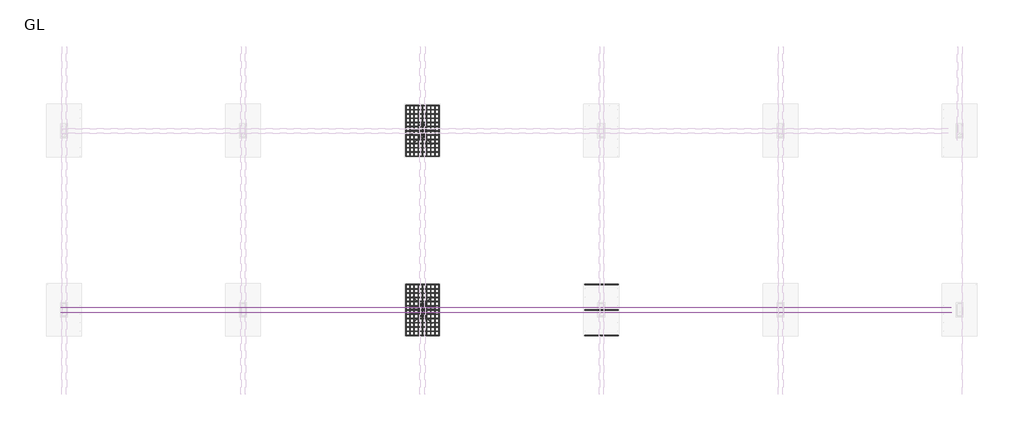
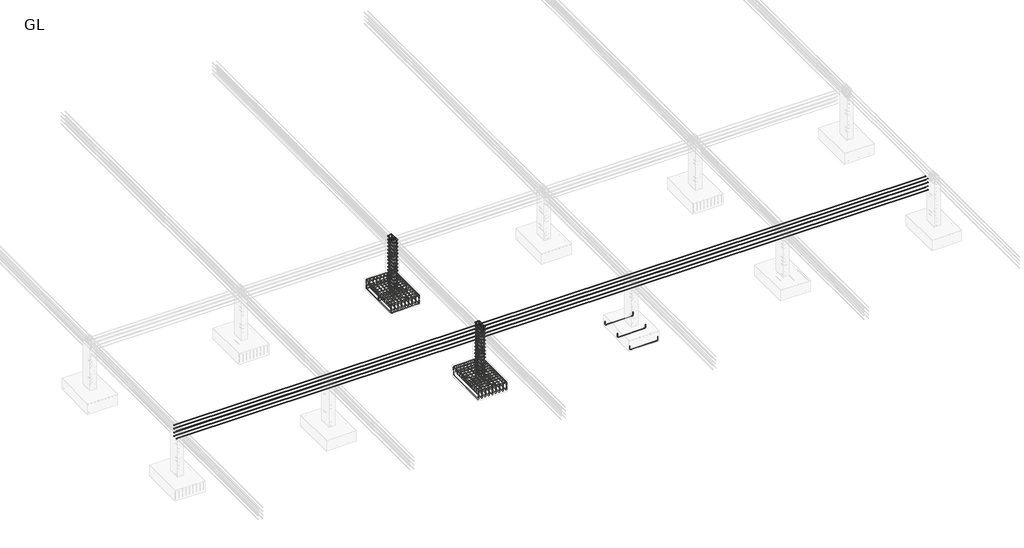
# One storey, part 7 of 16: 22 reinforcing bars.
"""IFC4 building model written with IfcOpenShell, lengths in millimetres."""

from ifc_helpers import new_model, si_unit, point, frame, origin, place, context, project, spatial, polyline, circle_curve, trimmed, segment, composite_curve, source, transform, mapped, element, save
from ifc_brep_helpers import swept_disk

model = new_model("IFC4")

# Units and contexts
model_context = context("Model", 3, world=origin())
ifc_project = project(units=[si_unit("LENGTHUNIT", "METRE", prefix="MILLI")], contexts=[model_context])

# Site, building, storey
site = spatial("IfcSite", under=ifc_project)
building = spatial("IfcBuilding", under=site)
storey = spatial("IfcBuildingStorey", under=building, Name="GL", Elevation=-1829.0)

# Reinforcing bars
placement = place(None, origin())
reinforcing_bar_shape = source(origin(), model_context, "Body", "SolidModel", [
    swept_disk(composite_curve([segment(polyline([(-10050.9544379, -7223.1167521, -2089.0), (-10050.9544379, -7223.1167521, -2213.0)]), True, "CONTINUOUS"), segment(trimmed(circle_curve(frame((-10080.9544379, -7223.1167521, -2213.0), z_axis=(0.0, 1.0, 0.0), x_axis=(30.0, 0.0, 0.0)), 30.0), [point((-10050.9544379, -7223.1167521, -2213.0))], [point((-10080.9544379, -7223.1167521, -2243.0))], True, "CARTESIAN"), True, "CONTINUOUS"), segment(polyline([(-10080.9544379, -7223.1167521, -2243.0), (-11148.9544379, -7223.1167521, -2243.0)]), True, "CONTINUOUS"), segment(trimmed(circle_curve(frame((-11148.9544379, -7223.1167521, -2213.0), z_axis=(0.0, 1.0, 0.0), x_axis=(0.0, 0.0, -30.0)), 30.0), [point((-11148.9544379, -7223.1167521, -2243.0))], [point((-11178.9544379, -7223.1167521, -2213.0))], True, "CARTESIAN"), True, "CONTINUOUS"), segment(polyline([(-11178.9544379, -7223.1167521, -2213.0), (-11178.9544379, -7223.1167521, -2089.0)]), True, "CONTINUOUS")], self_intersect=False), 6.0),
])
element("IfcReinforcingBar", 1, at=placement, inside=storey, context=model_context, shape_type="MappedRepresentation", body=[
    mapped(reinforcing_bar_shape, transform((0.0, 0.0, 0.0), x_axis=(1.0, 0.0, 0.0), y_axis=(0.0, 1.0, 0.0), z_axis=(0.0, 0.0, 1.0))),
    mapped(reinforcing_bar_shape, transform((0.0, -864.0, 0.0), x_axis=(1.0, 0.0, 0.0), y_axis=(0.0, 1.0, 0.0), z_axis=(0.0, 0.0, 1.0))),
    mapped(reinforcing_bar_shape, transform((0.0, -1728.0, 0.0), x_axis=(1.0, 0.0, 0.0), y_axis=(0.0, 1.0, 0.0), z_axis=(0.0, 0.0, 1.0))),
])
reinforcing_bar_2_shape = source(origin(), model_context, "Body", "SolidModel", [
    swept_disk(composite_curve([segment(polyline([(-11178.9544379, -7223.1167521, -2022.436678), (-11178.9544379, -7223.1167521, -1898.436678)]), True, "CONTINUOUS"), segment(trimmed(circle_curve(frame((-11148.9544379, -7223.1167521, -1898.436678), z_axis=(0.0, 1.0, 0.0), x_axis=(-30.0, 0.0, 0.0)), 30.0), [point((-11178.9544379, -7223.1167521, -1898.436678))], [point((-11148.9544379, -7223.1167521, -1868.436678))], True, "CARTESIAN"), True, "CONTINUOUS"), segment(polyline([(-11148.9544379, -7223.1167521, -1868.436678), (-10080.9544379, -7223.1167521, -1868.436678)]), True, "CONTINUOUS"), segment(trimmed(circle_curve(frame((-10080.9544379, -7223.1167521, -1898.436678), z_axis=(0.0, 1.0, 0.0), x_axis=(0.0, 0.0, 30.0)), 30.0), [point((-10080.9544379, -7223.1167521, -1868.436678))], [point((-10050.9544379, -7223.1167521, -1898.436678))], True, "CARTESIAN"), True, "CONTINUOUS"), segment(polyline([(-10050.9544379, -7223.1167521, -1898.436678), (-10050.9544379, -7223.1167521, -2022.436678)]), True, "CONTINUOUS")], self_intersect=False), 6.0),
])
element("IfcReinforcingBar", 2, at=placement, inside=storey, context=model_context, shape_type="MappedRepresentation", body=[
    mapped(reinforcing_bar_2_shape, transform((0.0, 0.0, 0.0), x_axis=(1.0, 0.0, 0.0), y_axis=(0.0, 1.0, 0.0), z_axis=(0.0, 0.0, 1.0))),
    mapped(reinforcing_bar_2_shape, transform((0.0, -144.0, 0.0), x_axis=(1.0, 0.0, 0.0), y_axis=(0.0, 1.0, 0.0), z_axis=(0.0, 0.0, 1.0))),
    mapped(reinforcing_bar_2_shape, transform((0.0, -288.0, 0.0), x_axis=(1.0, 0.0, 0.0), y_axis=(0.0, 1.0, 0.0), z_axis=(0.0, 0.0, 1.0))),
    mapped(reinforcing_bar_2_shape, transform((0.0, -432.0, 0.0), x_axis=(1.0, 0.0, 0.0), y_axis=(0.0, 1.0, 0.0), z_axis=(0.0, 0.0, 1.0))),
    mapped(reinforcing_bar_2_shape, transform((0.0, -576.0, 0.0), x_axis=(1.0, 0.0, 0.0), y_axis=(0.0, 1.0, 0.0), z_axis=(0.0, 0.0, 1.0))),
    mapped(reinforcing_bar_2_shape, transform((0.0, -720.0, 0.0), x_axis=(1.0, 0.0, 0.0), y_axis=(0.0, 1.0, 0.0), z_axis=(0.0, 0.0, 1.0))),
    mapped(reinforcing_bar_2_shape, transform((0.0, -864.0, 0.0), x_axis=(1.0, 0.0, 0.0), y_axis=(0.0, 1.0, 0.0), z_axis=(0.0, 0.0, 1.0))),
    mapped(reinforcing_bar_2_shape, transform((0.0, -1008.0, 0.0), x_axis=(1.0, 0.0, 0.0), y_axis=(0.0, 1.0, 0.0), z_axis=(0.0, 0.0, 1.0))),
    mapped(reinforcing_bar_2_shape, transform((0.0, -1152.0, 0.0), x_axis=(1.0, 0.0, 0.0), y_axis=(0.0, 1.0, 0.0), z_axis=(0.0, 0.0, 1.0))),
    mapped(reinforcing_bar_2_shape, transform((0.0, -1296.0, 0.0), x_axis=(1.0, 0.0, 0.0), y_axis=(0.0, 1.0, 0.0), z_axis=(0.0, 0.0, 1.0))),
    mapped(reinforcing_bar_2_shape, transform((0.0, -1440.0, 0.0), x_axis=(1.0, 0.0, 0.0), y_axis=(0.0, 1.0, 0.0), z_axis=(0.0, 0.0, 1.0))),
    mapped(reinforcing_bar_2_shape, transform((0.0, -1584.0, 0.0), x_axis=(1.0, 0.0, 0.0), y_axis=(0.0, 1.0, 0.0), z_axis=(0.0, 0.0, 1.0))),
    mapped(reinforcing_bar_2_shape, transform((0.0, -1728.0, 0.0), x_axis=(1.0, 0.0, 0.0), y_axis=(0.0, 1.0, 0.0), z_axis=(0.0, 0.0, 1.0))),
])
reinforcing_bar_3_shape = source(origin(), model_context, "Body", "SolidModel", [
    swept_disk(composite_curve([segment(polyline([(-11178.9544379, -8951.1167521, -2027.5081232), (-11178.9544379, -8951.1167521, -1903.5081232)]), True, "CONTINUOUS"), segment(trimmed(circle_curve(frame((-11178.9544379, -8921.1167521, -1903.5081232), z_axis=(-1.0, 0.0, 0.0), x_axis=(0.0, -30.0, 0.0)), 30.0), [point((-11178.9544379, -8951.1167521, -1903.5081232))], [point((-11178.9544379, -8921.1167521, -1873.5081232))], True, "CARTESIAN"), True, "CONTINUOUS"), segment(polyline([(-11178.9544379, -8921.1167521, -1873.5081232), (-11178.9544379, -7253.1167521, -1873.5081232)]), True, "CONTINUOUS"), segment(trimmed(circle_curve(frame((-11178.9544379, -7253.1167521, -1903.5081232), z_axis=(-1.0, 0.0, 0.0), x_axis=(0.0, 0.0, 30.0)), 30.0), [point((-11178.9544379, -7253.1167521, -1873.5081232))], [point((-11178.9544379, -7223.1167521, -1903.5081232))], True, "CARTESIAN"), True, "CONTINUOUS"), segment(polyline([(-11178.9544379, -7223.1167521, -1903.5081232), (-11178.9544379, -7223.1167521, -2027.5081232)]), True, "CONTINUOUS")], self_intersect=False), 6.0),
])
element("IfcReinforcingBar", 3, at=placement, inside=storey, context=model_context, shape_type="MappedRepresentation", body=[
    mapped(reinforcing_bar_3_shape, transform((0.0, 0.0, 0.0), x_axis=(1.0, 0.0, 0.0), y_axis=(0.0, 1.0, 0.0), z_axis=(0.0, 0.0, 1.0))),
    mapped(reinforcing_bar_3_shape, transform((141.0, 0.0, 0.0), x_axis=(1.0, 0.0, 0.0), y_axis=(0.0, 1.0, 0.0), z_axis=(0.0, 0.0, 1.0))),
    mapped(reinforcing_bar_3_shape, transform((282.0, 0.0, 0.0), x_axis=(1.0, 0.0, 0.0), y_axis=(0.0, 1.0, 0.0), z_axis=(0.0, 0.0, 1.0))),
    mapped(reinforcing_bar_3_shape, transform((423.0, 0.0, 0.0), x_axis=(1.0, 0.0, 0.0), y_axis=(0.0, 1.0, 0.0), z_axis=(0.0, 0.0, 1.0))),
    mapped(reinforcing_bar_3_shape, transform((564.0, 0.0, 0.0), x_axis=(1.0, 0.0, 0.0), y_axis=(0.0, 1.0, 0.0), z_axis=(0.0, 0.0, 1.0))),
    mapped(reinforcing_bar_3_shape, transform((705.0, 0.0, 0.0), x_axis=(1.0, 0.0, 0.0), y_axis=(0.0, 1.0, 0.0), z_axis=(0.0, 0.0, 1.0))),
    mapped(reinforcing_bar_3_shape, transform((846.0, 0.0, 0.0), x_axis=(1.0, 0.0, 0.0), y_axis=(0.0, 1.0, 0.0), z_axis=(0.0, 0.0, 1.0))),
    mapped(reinforcing_bar_3_shape, transform((987.0, 0.0, 0.0), x_axis=(1.0, 0.0, 0.0), y_axis=(0.0, 1.0, 0.0), z_axis=(0.0, 0.0, 1.0))),
    mapped(reinforcing_bar_3_shape, transform((1128.0, 0.0, 0.0), x_axis=(1.0, 0.0, 0.0), y_axis=(0.0, 1.0, 0.0), z_axis=(0.0, 0.0, 1.0))),
])
reinforcing_bar_4_shape = source(origin(), model_context, "Body", "SolidModel", [
    swept_disk(composite_curve([segment(polyline([(-10050.9544379, -8951.1167521, -2080.6239909), (-10050.9544379, -8951.1167521, -2204.6239909)]), True, "CONTINUOUS"), segment(trimmed(circle_curve(frame((-10050.9544379, -8921.1167521, -2204.6239909), z_axis=(1.0, 0.0, 0.0), x_axis=(0.0, -30.0, 0.0)), 30.0), [point((-10050.9544379, -8951.1167521, -2204.6239909))], [point((-10050.9544379, -8921.1167521, -2234.6239909))], True, "CARTESIAN"), True, "CONTINUOUS"), segment(polyline([(-10050.9544379, -8921.1167521, -2234.6239909), (-10050.9544379, -7266.1421892, -2234.6239909)]), True, "CONTINUOUS"), segment(trimmed(circle_curve(frame((-10050.9544379, -7266.1421892, -2204.6239909), z_axis=(1.0, 0.0, 0.0), x_axis=(0.0, 0.0, -30.0)), 30.0), [point((-10050.9544379, -7266.1421892, -2234.6239909))], [point((-10050.9544379, -7236.1421892, -2204.6239909))], True, "CARTESIAN"), True, "CONTINUOUS"), segment(polyline([(-10050.9544379, -7236.1421892, -2204.6239909), (-10050.9544379, -7236.1421892, -2080.6239909)]), True, "CONTINUOUS")], self_intersect=False), 6.0),
])
element("IfcReinforcingBar", 4, at=placement, inside=storey, context=model_context, shape_type="MappedRepresentation", body=[
    mapped(reinforcing_bar_4_shape, transform((0.0, 0.0, 0.0), x_axis=(1.0, 0.0, 0.0), y_axis=(0.0, 1.0, 0.0), z_axis=(0.0, 0.0, 1.0))),
    mapped(reinforcing_bar_4_shape, transform((-141.0, 0.0, 0.0), x_axis=(1.0, 0.0, 0.0), y_axis=(0.0, 1.0, 0.0), z_axis=(0.0, 0.0, 1.0))),
    mapped(reinforcing_bar_4_shape, transform((-282.0, 0.0, 0.0), x_axis=(1.0, 0.0, 0.0), y_axis=(0.0, 1.0, 0.0), z_axis=(0.0, 0.0, 1.0))),
    mapped(reinforcing_bar_4_shape, transform((-423.0, 0.0, 0.0), x_axis=(1.0, 0.0, 0.0), y_axis=(0.0, 1.0, 0.0), z_axis=(0.0, 0.0, 1.0))),
    mapped(reinforcing_bar_4_shape, transform((-564.0, 0.0, 0.0), x_axis=(1.0, 0.0, 0.0), y_axis=(0.0, 1.0, 0.0), z_axis=(0.0, 0.0, 1.0))),
    mapped(reinforcing_bar_4_shape, transform((-705.0, 0.0, 0.0), x_axis=(1.0, 0.0, 0.0), y_axis=(0.0, 1.0, 0.0), z_axis=(0.0, 0.0, 1.0))),
    mapped(reinforcing_bar_4_shape, transform((-846.0, 0.0, 0.0), x_axis=(1.0, 0.0, 0.0), y_axis=(0.0, 1.0, 0.0), z_axis=(0.0, 0.0, 1.0))),
    mapped(reinforcing_bar_4_shape, transform((-987.0, 0.0, 0.0), x_axis=(1.0, 0.0, 0.0), y_axis=(0.0, 1.0, 0.0), z_axis=(0.0, 0.0, 1.0))),
    mapped(reinforcing_bar_4_shape, transform((-1128.0, 0.0, 0.0), x_axis=(1.0, 0.0, 0.0), y_axis=(0.0, 1.0, 0.0), z_axis=(0.0, 0.0, 1.0))),
])
reinforcing_bar_5_shape = source(origin(), model_context, "Body", "SolidModel", [
    swept_disk(composite_curve([segment(polyline([(-3954.9544379, -13319.1167521, -2089.0), (-3954.9544379, -13319.1167521, -2213.0)]), True, "CONTINUOUS"), segment(trimmed(circle_curve(frame((-3984.9544379, -13319.1167521, -2213.0), z_axis=(0.0, 1.0, 0.0), x_axis=(30.0, 0.0, 0.0)), 30.0), [point((-3954.9544379, -13319.1167521, -2213.0))], [point((-3984.9544379, -13319.1167521, -2243.0))], True, "CARTESIAN"), True, "CONTINUOUS"), segment(polyline([(-3984.9544379, -13319.1167521, -2243.0), (-5052.9544379, -13319.1167521, -2243.0)]), True, "CONTINUOUS"), segment(trimmed(circle_curve(frame((-5052.9544379, -13319.1167521, -2213.0), z_axis=(0.0, 1.0, 0.0), x_axis=(0.0, 0.0, -30.0)), 30.0), [point((-5052.9544379, -13319.1167521, -2243.0))], [point((-5082.9544379, -13319.1167521, -2213.0))], True, "CARTESIAN"), True, "CONTINUOUS"), segment(polyline([(-5082.9544379, -13319.1167521, -2213.0), (-5082.9544379, -13319.1167521, -2089.0)]), True, "CONTINUOUS")], self_intersect=False), 6.0),
])
element("IfcReinforcingBar", 5, at=placement, inside=storey, context=model_context, shape_type="MappedRepresentation", body=[
    mapped(reinforcing_bar_5_shape, transform((0.0, 0.0, 0.0), x_axis=(1.0, 0.0, 0.0), y_axis=(0.0, 1.0, 0.0), z_axis=(0.0, 0.0, 1.0))),
    mapped(reinforcing_bar_5_shape, transform((0.0, -864.0, 0.0), x_axis=(1.0, 0.0, 0.0), y_axis=(0.0, 1.0, 0.0), z_axis=(0.0, 0.0, 1.0))),
    mapped(reinforcing_bar_5_shape, transform((0.0, -1728.0, 0.0), x_axis=(1.0, 0.0, 0.0), y_axis=(0.0, 1.0, 0.0), z_axis=(0.0, 0.0, 1.0))),
])
reinforcing_bar_6_shape = source(origin(), model_context, "Body", "SolidModel", [
    swept_disk(composite_curve([segment(polyline([(-11178.9544379, -13319.1167521, -2022.436678), (-11178.9544379, -13319.1167521, -1898.436678)]), True, "CONTINUOUS"), segment(trimmed(circle_curve(frame((-11148.9544379, -13319.1167521, -1898.436678), z_axis=(0.0, 1.0, 0.0), x_axis=(-30.0, 0.0, 0.0)), 30.0), [point((-11178.9544379, -13319.1167521, -1898.436678))], [point((-11148.9544379, -13319.1167521, -1868.436678))], True, "CARTESIAN"), True, "CONTINUOUS"), segment(polyline([(-11148.9544379, -13319.1167521, -1868.436678), (-10080.9544379, -13319.1167521, -1868.436678)]), True, "CONTINUOUS"), segment(trimmed(circle_curve(frame((-10080.9544379, -13319.1167521, -1898.436678), z_axis=(0.0, 1.0, 0.0), x_axis=(0.0, 0.0, 30.0)), 30.0), [point((-10080.9544379, -13319.1167521, -1868.436678))], [point((-10050.9544379, -13319.1167521, -1898.436678))], True, "CARTESIAN"), True, "CONTINUOUS"), segment(polyline([(-10050.9544379, -13319.1167521, -1898.436678), (-10050.9544379, -13319.1167521, -2022.436678)]), True, "CONTINUOUS")], self_intersect=False), 6.0),
])
element("IfcReinforcingBar", 6, at=placement, inside=storey, context=model_context, shape_type="MappedRepresentation", body=[
    mapped(reinforcing_bar_6_shape, transform((0.0, 0.0, 0.0), x_axis=(1.0, 0.0, 0.0), y_axis=(0.0, 1.0, 0.0), z_axis=(0.0, 0.0, 1.0))),
    mapped(reinforcing_bar_6_shape, transform((0.0, -144.0, 0.0), x_axis=(1.0, 0.0, 0.0), y_axis=(0.0, 1.0, 0.0), z_axis=(0.0, 0.0, 1.0))),
    mapped(reinforcing_bar_6_shape, transform((0.0, -288.0, 0.0), x_axis=(1.0, 0.0, 0.0), y_axis=(0.0, 1.0, 0.0), z_axis=(0.0, 0.0, 1.0))),
    mapped(reinforcing_bar_6_shape, transform((0.0, -432.0, 0.0), x_axis=(1.0, 0.0, 0.0), y_axis=(0.0, 1.0, 0.0), z_axis=(0.0, 0.0, 1.0))),
    mapped(reinforcing_bar_6_shape, transform((0.0, -576.0, 0.0), x_axis=(1.0, 0.0, 0.0), y_axis=(0.0, 1.0, 0.0), z_axis=(0.0, 0.0, 1.0))),
    mapped(reinforcing_bar_6_shape, transform((0.0, -720.0, 0.0), x_axis=(1.0, 0.0, 0.0), y_axis=(0.0, 1.0, 0.0), z_axis=(0.0, 0.0, 1.0))),
    mapped(reinforcing_bar_6_shape, transform((0.0, -864.0, 0.0), x_axis=(1.0, 0.0, 0.0), y_axis=(0.0, 1.0, 0.0), z_axis=(0.0, 0.0, 1.0))),
    mapped(reinforcing_bar_6_shape, transform((0.0, -1008.0, 0.0), x_axis=(1.0, 0.0, 0.0), y_axis=(0.0, 1.0, 0.0), z_axis=(0.0, 0.0, 1.0))),
    mapped(reinforcing_bar_6_shape, transform((0.0, -1152.0, 0.0), x_axis=(1.0, 0.0, 0.0), y_axis=(0.0, 1.0, 0.0), z_axis=(0.0, 0.0, 1.0))),
    mapped(reinforcing_bar_6_shape, transform((0.0, -1296.0, 0.0), x_axis=(1.0, 0.0, 0.0), y_axis=(0.0, 1.0, 0.0), z_axis=(0.0, 0.0, 1.0))),
    mapped(reinforcing_bar_6_shape, transform((0.0, -1440.0, 0.0), x_axis=(1.0, 0.0, 0.0), y_axis=(0.0, 1.0, 0.0), z_axis=(0.0, 0.0, 1.0))),
    mapped(reinforcing_bar_6_shape, transform((0.0, -1584.0, 0.0), x_axis=(1.0, 0.0, 0.0), y_axis=(0.0, 1.0, 0.0), z_axis=(0.0, 0.0, 1.0))),
    mapped(reinforcing_bar_6_shape, transform((0.0, -1728.0, 0.0), x_axis=(1.0, 0.0, 0.0), y_axis=(0.0, 1.0, 0.0), z_axis=(0.0, 0.0, 1.0))),
])
reinforcing_bar_7_shape = source(origin(), model_context, "Body", "SolidModel", [
    swept_disk(composite_curve([segment(polyline([(-11178.9544379, -15047.1167521, -2027.5081232), (-11178.9544379, -15047.1167521, -1903.5081232)]), True, "CONTINUOUS"), segment(trimmed(circle_curve(frame((-11178.9544379, -15017.1167521, -1903.5081232), z_axis=(-1.0, 0.0, 0.0), x_axis=(0.0, -30.0, 0.0)), 30.0), [point((-11178.9544379, -15047.1167521, -1903.5081232))], [point((-11178.9544379, -15017.1167521, -1873.5081232))], True, "CARTESIAN"), True, "CONTINUOUS"), segment(polyline([(-11178.9544379, -15017.1167521, -1873.5081232), (-11178.9544379, -13349.1167521, -1873.5081232)]), True, "CONTINUOUS"), segment(trimmed(circle_curve(frame((-11178.9544379, -13349.1167521, -1903.5081232), z_axis=(-1.0, 0.0, 0.0), x_axis=(0.0, 0.0, 30.0)), 30.0), [point((-11178.9544379, -13349.1167521, -1873.5081232))], [point((-11178.9544379, -13319.1167521, -1903.5081232))], True, "CARTESIAN"), True, "CONTINUOUS"), segment(polyline([(-11178.9544379, -13319.1167521, -1903.5081232), (-11178.9544379, -13319.1167521, -2027.5081232)]), True, "CONTINUOUS")], self_intersect=False), 6.0),
])
element("IfcReinforcingBar", 7, at=placement, inside=storey, context=model_context, shape_type="MappedRepresentation", body=[
    mapped(reinforcing_bar_7_shape, transform((0.0, 0.0, 0.0), x_axis=(1.0, 0.0, 0.0), y_axis=(0.0, 1.0, 0.0), z_axis=(0.0, 0.0, 1.0))),
    mapped(reinforcing_bar_7_shape, transform((141.0, 0.0, 0.0), x_axis=(1.0, 0.0, 0.0), y_axis=(0.0, 1.0, 0.0), z_axis=(0.0, 0.0, 1.0))),
    mapped(reinforcing_bar_7_shape, transform((282.0, 0.0, 0.0), x_axis=(1.0, 0.0, 0.0), y_axis=(0.0, 1.0, 0.0), z_axis=(0.0, 0.0, 1.0))),
    mapped(reinforcing_bar_7_shape, transform((423.0, 0.0, 0.0), x_axis=(1.0, 0.0, 0.0), y_axis=(0.0, 1.0, 0.0), z_axis=(0.0, 0.0, 1.0))),
    mapped(reinforcing_bar_7_shape, transform((564.0, 0.0, 0.0), x_axis=(1.0, 0.0, 0.0), y_axis=(0.0, 1.0, 0.0), z_axis=(0.0, 0.0, 1.0))),
    mapped(reinforcing_bar_7_shape, transform((705.0, 0.0, 0.0), x_axis=(1.0, 0.0, 0.0), y_axis=(0.0, 1.0, 0.0), z_axis=(0.0, 0.0, 1.0))),
    mapped(reinforcing_bar_7_shape, transform((846.0, 0.0, 0.0), x_axis=(1.0, 0.0, 0.0), y_axis=(0.0, 1.0, 0.0), z_axis=(0.0, 0.0, 1.0))),
    mapped(reinforcing_bar_7_shape, transform((987.0, 0.0, 0.0), x_axis=(1.0, 0.0, 0.0), y_axis=(0.0, 1.0, 0.0), z_axis=(0.0, 0.0, 1.0))),
    mapped(reinforcing_bar_7_shape, transform((1128.0, 0.0, 0.0), x_axis=(1.0, 0.0, 0.0), y_axis=(0.0, 1.0, 0.0), z_axis=(0.0, 0.0, 1.0))),
])
reinforcing_bar_8_shape = source(origin(), model_context, "Body", "SolidModel", [
    swept_disk(composite_curve([segment(polyline([(-10050.9544379, -15047.1167521, -2080.6239909), (-10050.9544379, -15047.1167521, -2204.6239909)]), True, "CONTINUOUS"), segment(trimmed(circle_curve(frame((-10050.9544379, -15017.1167521, -2204.6239909), z_axis=(1.0, 0.0, 0.0), x_axis=(0.0, -30.0, 0.0)), 30.0), [point((-10050.9544379, -15047.1167521, -2204.6239909))], [point((-10050.9544379, -15017.1167521, -2234.6239909))], True, "CARTESIAN"), True, "CONTINUOUS"), segment(polyline([(-10050.9544379, -15017.1167521, -2234.6239909), (-10050.9544379, -13362.1421892, -2234.6239909)]), True, "CONTINUOUS"), segment(trimmed(circle_curve(frame((-10050.9544379, -13362.1421892, -2204.6239909), z_axis=(1.0, 0.0, 0.0), x_axis=(0.0, 0.0, -30.0)), 30.0), [point((-10050.9544379, -13362.1421892, -2234.6239909))], [point((-10050.9544379, -13332.1421892, -2204.6239909))], True, "CARTESIAN"), True, "CONTINUOUS"), segment(polyline([(-10050.9544379, -13332.1421892, -2204.6239909), (-10050.9544379, -13332.1421892, -2080.6239909)]), True, "CONTINUOUS")], self_intersect=False), 6.0),
])
element("IfcReinforcingBar", 8, at=placement, inside=storey, context=model_context, shape_type="MappedRepresentation", body=[
    mapped(reinforcing_bar_8_shape, transform((0.0, 0.0, 0.0), x_axis=(1.0, 0.0, 0.0), y_axis=(0.0, 1.0, 0.0), z_axis=(0.0, 0.0, 1.0))),
    mapped(reinforcing_bar_8_shape, transform((-141.0, 0.0, 0.0), x_axis=(1.0, 0.0, 0.0), y_axis=(0.0, 1.0, 0.0), z_axis=(0.0, 0.0, 1.0))),
    mapped(reinforcing_bar_8_shape, transform((-282.0, 0.0, 0.0), x_axis=(1.0, 0.0, 0.0), y_axis=(0.0, 1.0, 0.0), z_axis=(0.0, 0.0, 1.0))),
    mapped(reinforcing_bar_8_shape, transform((-423.0, 0.0, 0.0), x_axis=(1.0, 0.0, 0.0), y_axis=(0.0, 1.0, 0.0), z_axis=(0.0, 0.0, 1.0))),
    mapped(reinforcing_bar_8_shape, transform((-564.0, 0.0, 0.0), x_axis=(1.0, 0.0, 0.0), y_axis=(0.0, 1.0, 0.0), z_axis=(0.0, 0.0, 1.0))),
    mapped(reinforcing_bar_8_shape, transform((-705.0, 0.0, 0.0), x_axis=(1.0, 0.0, 0.0), y_axis=(0.0, 1.0, 0.0), z_axis=(0.0, 0.0, 1.0))),
    mapped(reinforcing_bar_8_shape, transform((-846.0, 0.0, 0.0), x_axis=(1.0, 0.0, 0.0), y_axis=(0.0, 1.0, 0.0), z_axis=(0.0, 0.0, 1.0))),
    mapped(reinforcing_bar_8_shape, transform((-987.0, 0.0, 0.0), x_axis=(1.0, 0.0, 0.0), y_axis=(0.0, 1.0, 0.0), z_axis=(0.0, 0.0, 1.0))),
    mapped(reinforcing_bar_8_shape, transform((-1128.0, 0.0, 0.0), x_axis=(1.0, 0.0, 0.0), y_axis=(0.0, 1.0, 0.0), z_axis=(0.0, 0.0, 1.0))),
])
reinforcing_bar_9_shape = source(origin(), model_context, "Body", "SolidModel", [
    swept_disk(composite_curve([segment(polyline([(-10607.4864005, -14258.2223078, -1793.0), (-10695.1676414, -14345.9035486, -1793.0)]), True, "CONTINUOUS"), segment(trimmed(circle_curve(frame((-10673.9544379, -14367.1167521, -1793.0), z_axis=(0.0, 0.0, 1.0), x_axis=(-21.21320349999951, 21.213203500001327, 0.0)), 30.0), [point((-10695.1676414, -14345.9035486, -1793.0))], [point((-10673.9544379, -14397.1167521, -1793.0))], True, "CARTESIAN"), True, "CONTINUOUS"), segment(polyline([(-10673.9544379, -14397.1167521, -1793.0), (-10555.9544379, -14397.1167521, -1793.0)]), True, "CONTINUOUS"), segment(trimmed(circle_curve(frame((-10555.9544379, -14367.1167521, -1793.0), z_axis=(0.0, 0.0, 1.0), x_axis=(0.0, -30.0, 0.0)), 30.0), [point((-10555.9544379, -14397.1167521, -1793.0))], [point((-10525.9544379, -14367.1167521, -1793.0))], True, "CARTESIAN"), True, "CONTINUOUS"), segment(polyline([(-10525.9544379, -14367.1167521, -1793.0), (-10525.9544379, -13999.1167521, -1793.0)]), True, "CONTINUOUS"), segment(trimmed(circle_curve(frame((-10555.8864962, -13999.1167521, -1795.0178916), z_axis=(-0.06726305234213417, 0.0, 0.9977352764083365), x_axis=(29.93205830000079, 0.0, 2.0178915999999845)), 30.0), [point((-10525.9544379, -13999.1167521, -1793.0))], [point((-10555.8864962, -13969.1167521, -1795.0178916))], True, "CARTESIAN"), True, "CONTINUOUS"), segment(polyline([(-10555.8864962, -13969.1167521, -1795.0178916), (-10674.0223796, -13969.1167521, -1802.9821084)]), True, "CONTINUOUS"), segment(trimmed(circle_curve(frame((-10674.0223796, -13999.1167521, -1802.9821084), z_axis=(-0.06726305234213417, 0.0, 0.9977352764083365), x_axis=(0.0, 30.0, 0.0)), 30.0), [point((-10674.0223796, -13969.1167521, -1802.9821084))], [point((-10703.9544379, -13999.1167521, -1805.0))], True, "CARTESIAN"), True, "CONTINUOUS"), segment(polyline([(-10703.9544379, -13999.1167521, -1805.0), (-10703.9544379, -14367.1167521, -1805.0)]), True, "CONTINUOUS"), segment(trimmed(circle_curve(frame((-10673.9544379, -14367.1167521, -1805.0), z_axis=(0.0, 0.0, 1.0), x_axis=(-30.0, 0.0, 0.0)), 30.0), [point((-10703.9544379, -14367.1167521, -1805.0))], [point((-10652.7412345, -14388.3299555, -1805.0))], True, "CARTESIAN"), True, "CONTINUOUS"), segment(polyline([(-10652.7412345, -14388.3299555, -1805.0), (-10565.0599936, -14300.6487146, -1805.0)]), True, "CONTINUOUS")], self_intersect=False), 6.0),
])
element("IfcReinforcingBar", 9, at=placement, inside=storey, context=model_context, shape_type="MappedRepresentation", body=[
    mapped(reinforcing_bar_9_shape, transform((0.0, 0.0, 0.0), x_axis=(1.0, 0.0, 0.0), y_axis=(0.0, 1.0, 0.0), z_axis=(0.0, 0.0, 1.0))),
    mapped(reinforcing_bar_9_shape, transform((0.0, 0.0, 144.8571429), x_axis=(1.0, 0.0, 0.0), y_axis=(0.0, 1.0, 0.0), z_axis=(0.0, 0.0, 1.0))),
    mapped(reinforcing_bar_9_shape, transform((0.0, 0.0, 289.7142857), x_axis=(1.0, 0.0, 0.0), y_axis=(0.0, 1.0, 0.0), z_axis=(0.0, 0.0, 1.0))),
    mapped(reinforcing_bar_9_shape, transform((0.0, 0.0, 434.5714286), x_axis=(1.0, 0.0, 0.0), y_axis=(0.0, 1.0, 0.0), z_axis=(0.0, 0.0, 1.0))),
    mapped(reinforcing_bar_9_shape, transform((0.0, 0.0, 579.4285714), x_axis=(1.0, 0.0, 0.0), y_axis=(0.0, 1.0, 0.0), z_axis=(0.0, 0.0, 1.0))),
    mapped(reinforcing_bar_9_shape, transform((0.0, 0.0, 724.2857143), x_axis=(1.0, 0.0, 0.0), y_axis=(0.0, 1.0, 0.0), z_axis=(0.0, 0.0, 1.0))),
    mapped(reinforcing_bar_9_shape, transform((0.0, 0.0, 869.1428571), x_axis=(1.0, 0.0, 0.0), y_axis=(0.0, 1.0, 0.0), z_axis=(0.0, 0.0, 1.0))),
    mapped(reinforcing_bar_9_shape, transform((0.0, 0.0, 1014.0), x_axis=(1.0, 0.0, 0.0), y_axis=(0.0, 1.0, 0.0), z_axis=(0.0, 0.0, 1.0))),
    mapped(reinforcing_bar_9_shape, transform((0.0, 0.0, 1158.8571429), x_axis=(1.0, 0.0, 0.0), y_axis=(0.0, 1.0, 0.0), z_axis=(0.0, 0.0, 1.0))),
    mapped(reinforcing_bar_9_shape, transform((0.0, 0.0, 1303.7142857), x_axis=(1.0, 0.0, 0.0), y_axis=(0.0, 1.0, 0.0), z_axis=(0.0, 0.0, 1.0))),
    mapped(reinforcing_bar_9_shape, transform((0.0, 0.0, 1448.5714286), x_axis=(1.0, 0.0, 0.0), y_axis=(0.0, 1.0, 0.0), z_axis=(0.0, 0.0, 1.0))),
    mapped(reinforcing_bar_9_shape, transform((0.0, 0.0, 1593.4285714), x_axis=(1.0, 0.0, 0.0), y_axis=(0.0, 1.0, 0.0), z_axis=(0.0, 0.0, 1.0))),
    mapped(reinforcing_bar_9_shape, transform((0.0, 0.0, 1738.2857143), x_axis=(1.0, 0.0, 0.0), y_axis=(0.0, 1.0, 0.0), z_axis=(0.0, 0.0, 1.0))),
    mapped(reinforcing_bar_9_shape, transform((0.0, 0.0, 1883.1428571), x_axis=(1.0, 0.0, 0.0), y_axis=(0.0, 1.0, 0.0), z_axis=(0.0, 0.0, 1.0))),
    mapped(reinforcing_bar_9_shape, transform((0.0, 0.0, 2028.0), x_axis=(1.0, 0.0, 0.0), y_axis=(0.0, 1.0, 0.0), z_axis=(0.0, 0.0, 1.0))),
])
element("IfcReinforcingBar", 10, at=placement, inside=storey, context=model_context, shape_type="SolidModel", body=[
    swept_disk(composite_curve([segment(polyline([(-10672.0642232, -14368.0642439, 241.0), (-10672.0642232, -14368.0642439, -2129.0)]), True, "CONTINUOUS"), segment(trimmed(circle_curve(frame((-10693.2774266, -14389.2774473, -2129.0), z_axis=(-0.7071067811865187, 0.7071067811865764, 0.0), x_axis=(21.213203400000566, 21.213203400000566, 0.0)), 30.0), [point((-10672.0642232, -14368.0642439, -2129.0))], [point((-10693.2774266, -14389.2774473, -2159.0))], True, "CARTESIAN"), True, "CONTINUOUS"), segment(polyline([(-10693.2774266, -14389.2774473, -2159.0), (-10940.7648, -14636.7648207, -2159.0)]), True, "CONTINUOUS")], self_intersect=False), 6.0),
])
element("IfcReinforcingBar", 11, at=placement, inside=storey, context=model_context, shape_type="SolidModel", body=[
    swept_disk(composite_curve([segment(polyline([(-10672.0642232, -13998.1692603, 241.0), (-10672.0642232, -13998.1692603, -2129.0)]), True, "CONTINUOUS"), segment(trimmed(circle_curve(frame((-10693.2774266, -13976.9560568, -2129.0), z_axis=(0.7071067811865218, 0.7071067811865733, 0.0), x_axis=(21.213203400000566, -21.21320349999951, 0.0)), 30.0), [point((-10672.0642232, -13998.1692603, -2129.0))], [point((-10693.2774266, -13976.9560568, -2159.0))], True, "CARTESIAN"), True, "CONTINUOUS"), segment(polyline([(-10693.2774266, -13976.9560568, -2159.0), (-10940.7648, -13729.4686834, -2159.0)]), True, "CONTINUOUS")], self_intersect=False), 6.0),
])
element("IfcReinforcingBar", 12, at=placement, inside=storey, context=model_context, shape_type="SolidModel", body=[
    swept_disk(composite_curve([segment(polyline([(-10557.8446527, -14368.0642439, 241.0), (-10557.8446527, -14368.0642439, -2129.0)]), True, "CONTINUOUS"), segment(trimmed(circle_curve(frame((-10536.6314492, -14389.2774473, -2129.0), z_axis=(-0.7071067811865248, -0.7071067811865703, 0.0), x_axis=(-21.21320349999951, 21.213203400000566, 0.0)), 30.0), [point((-10557.8446527, -14368.0642439, -2129.0))], [point((-10536.6314492, -14389.2774473, -2159.0))], True, "CARTESIAN"), True, "CONTINUOUS"), segment(polyline([(-10536.6314492, -14389.2774473, -2159.0), (-10289.1440758, -14636.7648207, -2159.0)]), True, "CONTINUOUS")], self_intersect=False), 6.0),
])
element("IfcReinforcingBar", 13, at=placement, inside=storey, context=model_context, shape_type="SolidModel", body=[
    swept_disk(composite_curve([segment(polyline([(-10557.8446527, -13998.1692603, 241.0), (-10557.8446527, -13998.1692603, -2129.0)]), True, "CONTINUOUS"), segment(trimmed(circle_curve(frame((-10536.6314492, -13976.9560568, -2129.0), z_axis=(0.7071067811865157, -0.7071067811865794, 0.0), x_axis=(-21.21320349999951, -21.21320349999951, 0.0)), 30.0), [point((-10557.8446527, -13998.1692603, -2129.0))], [point((-10536.6314492, -13976.9560568, -2159.0))], True, "CARTESIAN"), True, "CONTINUOUS"), segment(polyline([(-10536.6314492, -13976.9560568, -2159.0), (-10289.1440758, -13729.4686834, -2159.0)]), True, "CONTINUOUS")], self_intersect=False), 6.0),
])
reinforcing_bar_10_shape = source(origin(), model_context, "Body", "SolidModel", [
    swept_disk(composite_curve([segment(polyline([(-10672.0642232, -14290.9117405, 241.0), (-10672.0642232, -14290.9117405, -2129.0)]), True, "CONTINUOUS"), segment(trimmed(circle_curve(frame((-10702.0642232, -14290.9117405, -2129.0), z_axis=(0.0, 1.0, 0.0), x_axis=(30.0, 0.0, 0.0)), 30.0), [point((-10672.0642232, -14290.9117405, -2129.0))], [point((-10702.0642232, -14290.9117405, -2159.0))], True, "CARTESIAN"), True, "CONTINUOUS"), segment(polyline([(-10702.0642232, -14290.9117405, -2159.0), (-11052.0642232, -14290.9117405, -2159.0)]), True, "CONTINUOUS")], self_intersect=False), 6.0),
])
element("IfcReinforcingBar", 14, at=placement, inside=storey, context=model_context, shape_type="MappedRepresentation", body=[
    mapped(reinforcing_bar_10_shape, transform((0.0, 0.0, 0.0), x_axis=(1.0, 0.0, 0.0), y_axis=(0.0, 1.0, 0.0), z_axis=(0.0, 0.0, 1.0))),
    mapped(reinforcing_bar_10_shape, transform((0.0, 123.5823926, 0.0), x_axis=(1.0, 0.0, 0.0), y_axis=(0.0, 1.0, 0.0), z_axis=(0.0, 0.0, 1.0))),
    mapped(reinforcing_bar_10_shape, transform((0.0, 247.1647853, 0.0), x_axis=(1.0, 0.0, 0.0), y_axis=(0.0, 1.0, 0.0), z_axis=(0.0, 0.0, 1.0))),
])
reinforcing_bar_11_shape = source(origin(), model_context, "Body", "SolidModel", [
    swept_disk(composite_curve([segment(polyline([(-10557.8446527, -14290.9117405, 241.0), (-10557.8446527, -14290.9117405, -2129.0)]), True, "CONTINUOUS"), segment(trimmed(circle_curve(frame((-10527.8446527, -14290.9117405, -2129.0), z_axis=(0.0, -1.0, 0.0), x_axis=(-30.0, 0.0, 0.0)), 30.0), [point((-10557.8446527, -14290.9117405, -2129.0))], [point((-10527.8446527, -14290.9117405, -2159.0))], True, "CARTESIAN"), True, "CONTINUOUS"), segment(polyline([(-10527.8446527, -14290.9117405, -2159.0), (-10177.8446527, -14290.9117405, -2159.0)]), True, "CONTINUOUS")], self_intersect=False), 6.0),
])
element("IfcReinforcingBar", 15, at=placement, inside=storey, context=model_context, shape_type="MappedRepresentation", body=[
    mapped(reinforcing_bar_11_shape, transform((0.0, 0.0, 0.0), x_axis=(1.0, 0.0, 0.0), y_axis=(0.0, 1.0, 0.0), z_axis=(0.0, 0.0, 1.0))),
    mapped(reinforcing_bar_11_shape, transform((0.0, 123.5823926, 0.0), x_axis=(1.0, 0.0, 0.0), y_axis=(0.0, 1.0, 0.0), z_axis=(0.0, 0.0, 1.0))),
    mapped(reinforcing_bar_11_shape, transform((0.0, 247.1647853, 0.0), x_axis=(1.0, 0.0, 0.0), y_axis=(0.0, 1.0, 0.0), z_axis=(0.0, 0.0, 1.0))),
])
reinforcing_bar_12_shape = source(origin(), model_context, "Body", "SolidModel", [
    swept_disk(composite_curve([segment(polyline([(-10607.4864005, -8162.2223078, -1793.0), (-10695.1676414, -8249.9035486, -1793.0)]), True, "CONTINUOUS"), segment(trimmed(circle_curve(frame((-10673.9544379, -8271.1167521, -1793.0), z_axis=(0.0, 0.0, 1.0), x_axis=(-21.21320349999951, 21.213203500001327, 0.0)), 30.0), [point((-10695.1676414, -8249.9035486, -1793.0))], [point((-10673.9544379, -8301.1167521, -1793.0))], True, "CARTESIAN"), True, "CONTINUOUS"), segment(polyline([(-10673.9544379, -8301.1167521, -1793.0), (-10555.9544379, -8301.1167521, -1793.0)]), True, "CONTINUOUS"), segment(trimmed(circle_curve(frame((-10555.9544379, -8271.1167521, -1793.0), z_axis=(0.0, 0.0, 1.0), x_axis=(0.0, -30.0, 0.0)), 30.0), [point((-10555.9544379, -8301.1167521, -1793.0))], [point((-10525.9544379, -8271.1167521, -1793.0))], True, "CARTESIAN"), True, "CONTINUOUS"), segment(polyline([(-10525.9544379, -8271.1167521, -1793.0), (-10525.9544379, -7903.1167521, -1793.0)]), True, "CONTINUOUS"), segment(trimmed(circle_curve(frame((-10555.8864962, -7903.1167521, -1795.0178916), z_axis=(-0.06726305234213417, 0.0, 0.9977352764083365), x_axis=(29.93205830000079, 0.0, 2.0178915999999845)), 30.0), [point((-10525.9544379, -7903.1167521, -1793.0))], [point((-10555.8864962, -7873.1167521, -1795.0178916))], True, "CARTESIAN"), True, "CONTINUOUS"), segment(polyline([(-10555.8864962, -7873.1167521, -1795.0178916), (-10674.0223796, -7873.1167521, -1802.9821084)]), True, "CONTINUOUS"), segment(trimmed(circle_curve(frame((-10674.0223796, -7903.1167521, -1802.9821084), z_axis=(-0.06726305234213417, 0.0, 0.9977352764083365), x_axis=(0.0, 30.0, 0.0)), 30.0), [point((-10674.0223796, -7873.1167521, -1802.9821084))], [point((-10703.9544379, -7903.1167521, -1805.0))], True, "CARTESIAN"), True, "CONTINUOUS"), segment(polyline([(-10703.9544379, -7903.1167521, -1805.0), (-10703.9544379, -8271.1167521, -1805.0)]), True, "CONTINUOUS"), segment(trimmed(circle_curve(frame((-10673.9544379, -8271.1167521, -1805.0), z_axis=(0.0, 0.0, 1.0), x_axis=(-30.0, 0.0, 0.0)), 30.0), [point((-10703.9544379, -8271.1167521, -1805.0))], [point((-10652.7412345, -8292.3299555, -1805.0))], True, "CARTESIAN"), True, "CONTINUOUS"), segment(polyline([(-10652.7412345, -8292.3299555, -1805.0), (-10565.0599936, -8204.6487146, -1805.0)]), True, "CONTINUOUS")], self_intersect=False), 6.0),
])
element("IfcReinforcingBar", 16, at=placement, inside=storey, context=model_context, shape_type="MappedRepresentation", body=[
    mapped(reinforcing_bar_12_shape, transform((0.0, 0.0, 0.0), x_axis=(1.0, 0.0, 0.0), y_axis=(0.0, 1.0, 0.0), z_axis=(0.0, 0.0, 1.0))),
    mapped(reinforcing_bar_12_shape, transform((0.0, 0.0, 144.8571429), x_axis=(1.0, 0.0, 0.0), y_axis=(0.0, 1.0, 0.0), z_axis=(0.0, 0.0, 1.0))),
    mapped(reinforcing_bar_12_shape, transform((0.0, 0.0, 289.7142857), x_axis=(1.0, 0.0, 0.0), y_axis=(0.0, 1.0, 0.0), z_axis=(0.0, 0.0, 1.0))),
    mapped(reinforcing_bar_12_shape, transform((0.0, 0.0, 434.5714286), x_axis=(1.0, 0.0, 0.0), y_axis=(0.0, 1.0, 0.0), z_axis=(0.0, 0.0, 1.0))),
    mapped(reinforcing_bar_12_shape, transform((0.0, 0.0, 579.4285714), x_axis=(1.0, 0.0, 0.0), y_axis=(0.0, 1.0, 0.0), z_axis=(0.0, 0.0, 1.0))),
    mapped(reinforcing_bar_12_shape, transform((0.0, 0.0, 724.2857143), x_axis=(1.0, 0.0, 0.0), y_axis=(0.0, 1.0, 0.0), z_axis=(0.0, 0.0, 1.0))),
    mapped(reinforcing_bar_12_shape, transform((0.0, 0.0, 869.1428571), x_axis=(1.0, 0.0, 0.0), y_axis=(0.0, 1.0, 0.0), z_axis=(0.0, 0.0, 1.0))),
    mapped(reinforcing_bar_12_shape, transform((0.0, 0.0, 1014.0), x_axis=(1.0, 0.0, 0.0), y_axis=(0.0, 1.0, 0.0), z_axis=(0.0, 0.0, 1.0))),
    mapped(reinforcing_bar_12_shape, transform((0.0, 0.0, 1158.8571429), x_axis=(1.0, 0.0, 0.0), y_axis=(0.0, 1.0, 0.0), z_axis=(0.0, 0.0, 1.0))),
    mapped(reinforcing_bar_12_shape, transform((0.0, 0.0, 1303.7142857), x_axis=(1.0, 0.0, 0.0), y_axis=(0.0, 1.0, 0.0), z_axis=(0.0, 0.0, 1.0))),
    mapped(reinforcing_bar_12_shape, transform((0.0, 0.0, 1448.5714286), x_axis=(1.0, 0.0, 0.0), y_axis=(0.0, 1.0, 0.0), z_axis=(0.0, 0.0, 1.0))),
    mapped(reinforcing_bar_12_shape, transform((0.0, 0.0, 1593.4285714), x_axis=(1.0, 0.0, 0.0), y_axis=(0.0, 1.0, 0.0), z_axis=(0.0, 0.0, 1.0))),
    mapped(reinforcing_bar_12_shape, transform((0.0, 0.0, 1738.2857143), x_axis=(1.0, 0.0, 0.0), y_axis=(0.0, 1.0, 0.0), z_axis=(0.0, 0.0, 1.0))),
    mapped(reinforcing_bar_12_shape, transform((0.0, 0.0, 1883.1428571), x_axis=(1.0, 0.0, 0.0), y_axis=(0.0, 1.0, 0.0), z_axis=(0.0, 0.0, 1.0))),
    mapped(reinforcing_bar_12_shape, transform((0.0, 0.0, 2028.0), x_axis=(1.0, 0.0, 0.0), y_axis=(0.0, 1.0, 0.0), z_axis=(0.0, 0.0, 1.0))),
])
element("IfcReinforcingBar", 17, at=placement, inside=storey, context=model_context, shape_type="SolidModel", body=[
    swept_disk(composite_curve([segment(polyline([(-10672.0642232, -8272.0642439, 241.0), (-10672.0642232, -8272.0642439, -2129.0)]), True, "CONTINUOUS"), segment(trimmed(circle_curve(frame((-10693.2774266, -8293.2774473, -2129.0), z_axis=(-0.7071067811865187, 0.7071067811865764, 0.0), x_axis=(21.213203400000566, 21.213203400000566, 0.0)), 30.0), [point((-10672.0642232, -8272.0642439, -2129.0))], [point((-10693.2774266, -8293.2774473, -2159.0))], True, "CARTESIAN"), True, "CONTINUOUS"), segment(polyline([(-10693.2774266, -8293.2774473, -2159.0), (-10940.7648, -8540.7648207, -2159.0)]), True, "CONTINUOUS")], self_intersect=False), 6.0),
])
element("IfcReinforcingBar", 18, at=placement, inside=storey, context=model_context, shape_type="SolidModel", body=[
    swept_disk(composite_curve([segment(polyline([(-10557.8446527, -8272.0642439, 241.0), (-10557.8446527, -8272.0642439, -2129.0)]), True, "CONTINUOUS"), segment(trimmed(circle_curve(frame((-10536.6314492, -8293.2774473, -2129.0), z_axis=(-0.7071067811865248, -0.7071067811865703, 0.0), x_axis=(-21.21320349999951, 21.213203400000566, 0.0)), 30.0), [point((-10557.8446527, -8272.0642439, -2129.0))], [point((-10536.6314492, -8293.2774473, -2159.0))], True, "CARTESIAN"), True, "CONTINUOUS"), segment(polyline([(-10536.6314492, -8293.2774473, -2159.0), (-10289.1440758, -8540.7648207, -2159.0)]), True, "CONTINUOUS")], self_intersect=False), 6.0),
])
reinforcing_bar_13_shape = source(origin(), model_context, "Body", "SolidModel", [
    swept_disk(composite_curve([segment(polyline([(-10672.0642232, -8194.9117405, 241.0), (-10672.0642232, -8194.9117405, -2129.0)]), True, "CONTINUOUS"), segment(trimmed(circle_curve(frame((-10702.0642232, -8194.9117405, -2129.0), z_axis=(0.0, 1.0, 0.0), x_axis=(30.0, 0.0, 0.0)), 30.0), [point((-10672.0642232, -8194.9117405, -2129.0))], [point((-10702.0642232, -8194.9117405, -2159.0))], True, "CARTESIAN"), True, "CONTINUOUS"), segment(polyline([(-10702.0642232, -8194.9117405, -2159.0), (-11052.0642232, -8194.9117405, -2159.0)]), True, "CONTINUOUS")], self_intersect=False), 6.0),
])
element("IfcReinforcingBar", 19, at=placement, inside=storey, context=model_context, shape_type="MappedRepresentation", body=[
    mapped(reinforcing_bar_13_shape, transform((0.0, 0.0, 0.0), x_axis=(1.0, 0.0, 0.0), y_axis=(0.0, 1.0, 0.0), z_axis=(0.0, 0.0, 1.0))),
    mapped(reinforcing_bar_13_shape, transform((0.0, 123.5823926, 0.0), x_axis=(1.0, 0.0, 0.0), y_axis=(0.0, 1.0, 0.0), z_axis=(0.0, 0.0, 1.0))),
    mapped(reinforcing_bar_13_shape, transform((0.0, 247.1647853, 0.0), x_axis=(1.0, 0.0, 0.0), y_axis=(0.0, 1.0, 0.0), z_axis=(0.0, 0.0, 1.0))),
])
reinforcing_bar_14_shape = source(origin(), model_context, "Body", "SolidModel", [
    swept_disk(composite_curve([segment(polyline([(-10557.8446527, -8194.9117405, 241.0), (-10557.8446527, -8194.9117405, -2129.0)]), True, "CONTINUOUS"), segment(trimmed(circle_curve(frame((-10527.8446527, -8194.9117405, -2129.0), z_axis=(0.0, -1.0, 0.0), x_axis=(-30.0, 0.0, 0.0)), 30.0), [point((-10557.8446527, -8194.9117405, -2129.0))], [point((-10527.8446527, -8194.9117405, -2159.0))], True, "CARTESIAN"), True, "CONTINUOUS"), segment(polyline([(-10527.8446527, -8194.9117405, -2159.0), (-10177.8446527, -8194.9117405, -2159.0)]), True, "CONTINUOUS")], self_intersect=False), 6.0),
])
element("IfcReinforcingBar", 20, at=placement, inside=storey, context=model_context, shape_type="MappedRepresentation", body=[
    mapped(reinforcing_bar_14_shape, transform((0.0, 0.0, 0.0), x_axis=(1.0, 0.0, 0.0), y_axis=(0.0, 1.0, 0.0), z_axis=(0.0, 0.0, 1.0))),
    mapped(reinforcing_bar_14_shape, transform((0.0, 123.5823926, 0.0), x_axis=(1.0, 0.0, 0.0), y_axis=(0.0, 1.0, 0.0), z_axis=(0.0, 0.0, 1.0))),
    mapped(reinforcing_bar_14_shape, transform((0.0, 247.1647853, 0.0), x_axis=(1.0, 0.0, 0.0), y_axis=(0.0, 1.0, 0.0), z_axis=(0.0, 0.0, 1.0))),
])
reinforcing_bar_15_shape = source(origin(), model_context, "Body", "SolidModel", [
    swept_disk(composite_curve([segment(polyline([(7389.0128754, -14099.1167521, 206.4377006), (-22901.9544379, -14099.1167521, 206.4377006)]), True, "CONTINUOUS")], self_intersect=False), 6.0),
])
element("IfcReinforcingBar", 21, at=placement, inside=storey, context=model_context, shape_type="MappedRepresentation", body=[
    mapped(reinforcing_bar_15_shape, transform((0.0, 0.0, 0.0), x_axis=(1.0, 0.0, 0.0), y_axis=(0.0, 1.0, 0.0), z_axis=(0.0, 0.0, 1.0))),
    mapped(reinforcing_bar_15_shape, transform((0.0, 0.0, -158.800423), x_axis=(1.0, 0.0, 0.0), y_axis=(0.0, 1.0, 0.0), z_axis=(0.0, 0.0, 1.0))),
    mapped(reinforcing_bar_15_shape, transform((0.0, 0.0, -317.6008459), x_axis=(1.0, 0.0, 0.0), y_axis=(0.0, 1.0, 0.0), z_axis=(0.0, 0.0, 1.0))),
    mapped(reinforcing_bar_15_shape, transform((0.0, 0.0, -476.4012689), x_axis=(1.0, 0.0, 0.0), y_axis=(0.0, 1.0, 0.0), z_axis=(0.0, 0.0, 1.0))),
])
reinforcing_bar_16_shape = source(origin(), model_context, "Body", "SolidModel", [
    swept_disk(composite_curve([segment(polyline([(7390.3840456, -14267.1167521, -269.9635684), (-22901.9544379, -14267.1167521, -269.9635684)]), True, "CONTINUOUS")], self_intersect=False), 6.0),
])
element("IfcReinforcingBar", 22, at=placement, inside=storey, context=model_context, shape_type="MappedRepresentation", body=[
    mapped(reinforcing_bar_16_shape, transform((0.0, 0.0, 0.0), x_axis=(1.0, 0.0, 0.0), y_axis=(0.0, 1.0, 0.0), z_axis=(0.0, 0.0, 1.0))),
    mapped(reinforcing_bar_16_shape, transform((0.0, 0.0, 158.800423), x_axis=(1.0, 0.0, 0.0), y_axis=(0.0, 1.0, 0.0), z_axis=(0.0, 0.0, 1.0))),
    mapped(reinforcing_bar_16_shape, transform((0.0, 0.0, 317.6008459), x_axis=(1.0, 0.0, 0.0), y_axis=(0.0, 1.0, 0.0), z_axis=(0.0, 0.0, 1.0))),
    mapped(reinforcing_bar_16_shape, transform((0.0, 0.0, 476.4012689), x_axis=(1.0, 0.0, 0.0), y_axis=(0.0, 1.0, 0.0), z_axis=(0.0, 0.0, 1.0))),
])

save(model, "model.ifc")

# Revit data of these elements
# Elements 1, 2, 3, 4, 5, 6, 7, 8, 9, 10, 11, 12, 13, 14, 15, 16, 17, 18, 19, 20, 21, 22 (IfcReinforcingBar)
#   Phase Created = New Construction
